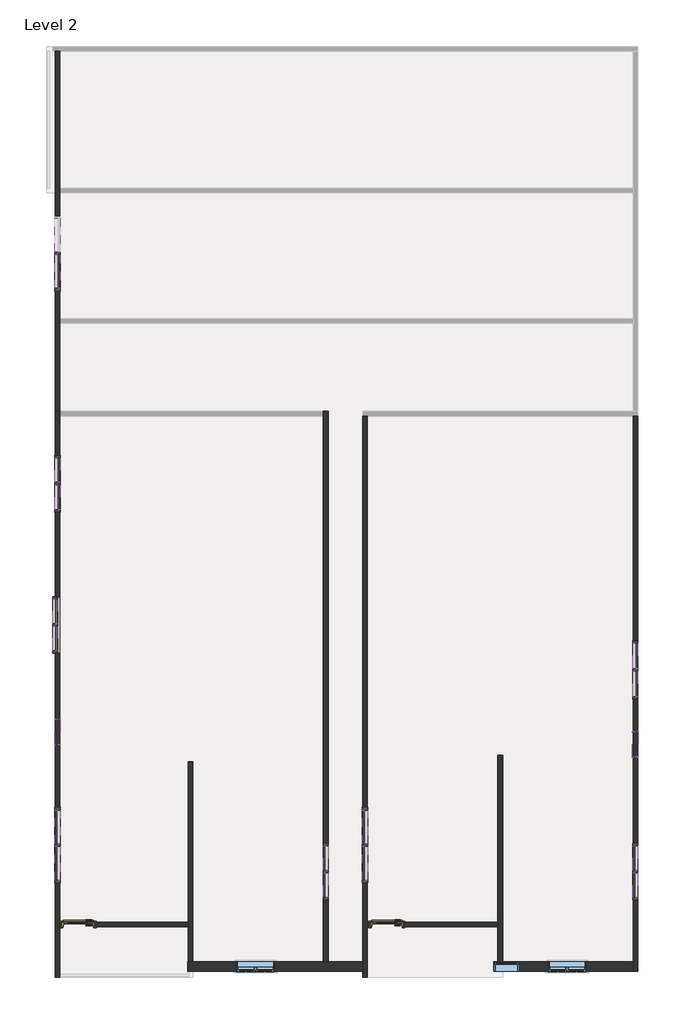
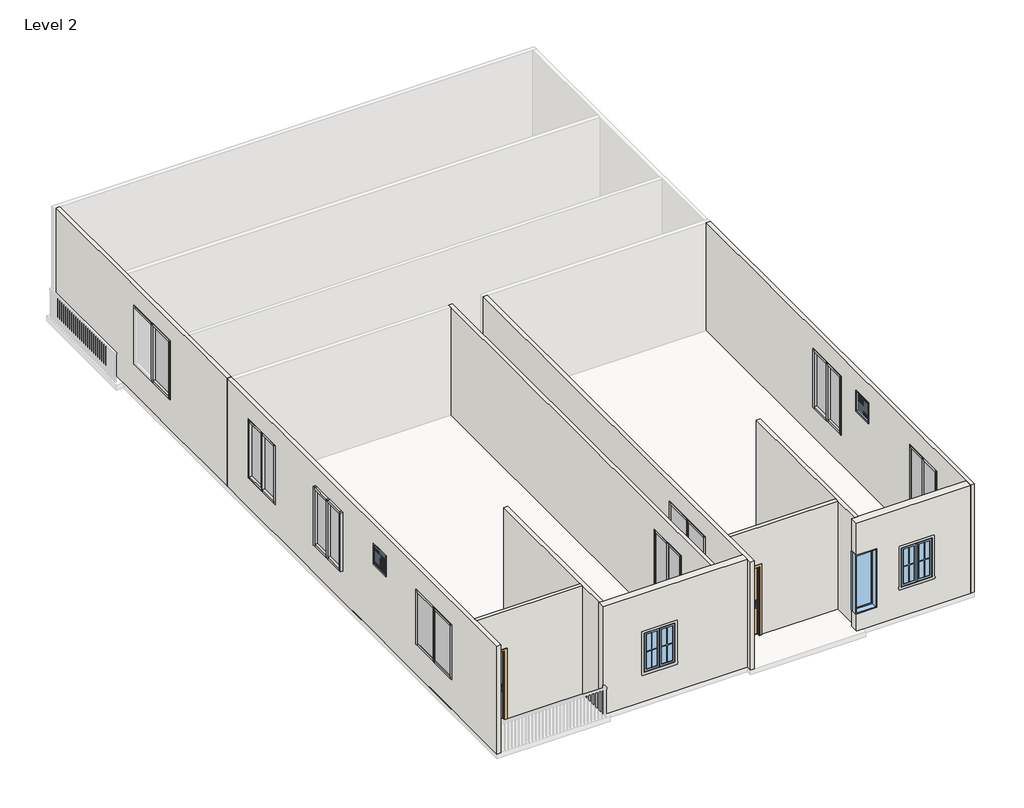
# One storey, part 1 of 2: 54 members, 15 plates, 11 walls, 5 windows, 2 doors.
"""IFC4 building model written with IfcOpenShell, lengths in millimetres."""

from ifc_helpers import new_model, si_unit, frame, origin, place, context, project, spatial, polyline, outline, extrude, faceted_brep, transform, mapped, element, save
from components import door_b81be692, member_8acf8d94, member_501b078b, member_3f0e0172, member_2e6d4a6b, member_96ae0c19, member_d60e8053, member_2fae0574, member_b8ac15de, member_17644e48, member_3e1d4a65, system_panel_glazed_c4393626, system_panel_glazed_0e71bc1b, system_panel_glazed_e97abd02, system_panel_glazed_d2c73f4b, system_panel_glazed_30879ba3, system_panel_glazed_a7ecbca6, window_fc882ab3, window_d341e8ac, window_d39e7ecb

model = new_model("IFC4")

# Units and contexts
model_context = context("Model", 3, world=origin())
ifc_project = project(units=[si_unit("LENGTHUNIT", "METRE", prefix="MILLI")], contexts=[model_context])

# Site, building, storey
site = spatial("IfcSite", under=ifc_project)
building = spatial("IfcBuilding", under=site)
storey = spatial("IfcBuildingStorey", under=building, Name="Level 2", Elevation=3352.8)

# Doors
placement = place(None, origin())
door_shape = door_b81be692(model_context)
element("IfcDoor", 1, ObjectType="29\" x 84\"", at=placement, inside=storey, context=model_context, shape_type="MappedRepresentation", body=[
    mapped(door_shape, transform((-7651.507583, -9448.7163489, 3352.8), x_axis=(1.0, 0.0, 0.0), y_axis=(0.0, 1.0, 0.0), z_axis=(0.0, 0.0, 1.0))),
])
element("IfcDoor", 2, ObjectType="29\" x 84\"", at=placement, inside=storey, context=model_context, shape_type="MappedRepresentation", body=[
    mapped(door_shape, transform((-172.2931282, -9448.9038009, 3352.8), x_axis=(1.0, 0.0, 0.0), y_axis=(0.0, 1.0, 0.0), z_axis=(0.0, 0.0, 1.0))),
])

# Members
member_shape = member_8acf8d94(model_context)
element("IfcMember", 3, ObjectType="Rectangular Mullion : 2.5\" x 5\" rectangular", at=placement, inside=storey, context=model_context, shape_type="MappedRepresentation", body=[
    mapped(member_shape, transform((-8153.157583, -8377.1401329, 5974.686558), x_axis=(0.0, 0.0, 1.0), y_axis=(-1.0, 0.0, 0.0), z_axis=(0.0, -1.0, 0.0))),
])
element("IfcMember", 4, ObjectType="Rectangular Mullion : 2.5\" x 5\" rectangular", at=placement, inside=storey, context=model_context, shape_type="MappedRepresentation", body=[
    mapped(member_shape, transform((-8153.157583, -7497.6651329, 5974.686558), x_axis=(0.0, 0.0, 1.0), y_axis=(-1.0, 0.0, 0.0), z_axis=(0.0, -1.0, 0.0))),
])
element("IfcMember", 5, ObjectType="Rectangular Mullion : 2.5\" x 5\" rectangular", at=placement, inside=storey, context=model_context, shape_type="MappedRepresentation", body=[
    mapped(member_shape, transform((-8153.157583, -6681.6901329, 4267.2), x_axis=(0.0, 0.0, -1.0), y_axis=(-1.0, 0.0, 0.0), z_axis=(0.0, 1.0, 0.0))),
])
element("IfcMember", 6, ObjectType="Rectangular Mullion : 2.5\" x 5\" rectangular", at=placement, inside=storey, context=model_context, shape_type="MappedRepresentation", body=[
    mapped(member_shape, transform((-8153.157583, -7561.1651329, 4267.2), x_axis=(0.0, 0.0, -1.0), y_axis=(-1.0, 0.0, 0.0), z_axis=(0.0, 1.0, 0.0))),
])
member_2_shape = member_501b078b(model_context)
element("IfcMember", 7, ObjectType="Rectangular Mullion : 2.5\" x 5\" rectangular", at=placement, inside=storey, context=model_context, shape_type="MappedRepresentation", body=[
    mapped(member_2_shape, transform((5848.1708786, -8795.0998253, 6096.0), x_axis=(0.0, 0.0, 1.0), y_axis=(-1.0, 0.0, 0.0), z_axis=(0.0, -1.0, 0.0))),
])
element("IfcMember", 8, ObjectType="Rectangular Mullion : 2.5\" x 5\" rectangular", at=placement, inside=storey, context=model_context, shape_type="MappedRepresentation", body=[
    mapped(member_2_shape, transform((5848.1708786, -8142.1745373, 6096.0), x_axis=(0.0, 0.0, 1.0), y_axis=(-1.0, 0.0, 0.0), z_axis=(0.0, -1.0, 0.0))),
])
element("IfcMember", 9, ObjectType="Rectangular Mullion : 2.5\" x 5\" rectangular", at=placement, inside=storey, context=model_context, shape_type="MappedRepresentation", body=[
    mapped(member_2_shape, transform((-1656.4435762, -8795.0998253, 6096.0), x_axis=(0.0, 0.0, 1.0), y_axis=(-1.0, 0.0, 0.0), z_axis=(0.0, -1.0, 0.0))),
])
element("IfcMember", 10, ObjectType="Rectangular Mullion : 2.5\" x 5\" rectangular", at=placement, inside=storey, context=model_context, shape_type="MappedRepresentation", body=[
    mapped(member_2_shape, transform((-1656.4435762, -8142.1745373, 6096.0), x_axis=(0.0, 0.0, 1.0), y_axis=(-1.0, 0.0, 0.0), z_axis=(0.0, -1.0, 0.0))),
])
element("IfcMember", 11, ObjectType="Rectangular Mullion : 2.5\" x 5\" rectangular", at=placement, inside=storey, context=model_context, shape_type="MappedRepresentation", body=[
    mapped(member_2_shape, transform((5848.1708786, -7552.7492493, 4267.2), x_axis=(0.0, 0.0, -1.0), y_axis=(-1.0, 0.0, 0.0), z_axis=(0.0, 1.0, 0.0))),
])
element("IfcMember", 12, ObjectType="Rectangular Mullion : 2.5\" x 5\" rectangular", at=placement, inside=storey, context=model_context, shape_type="MappedRepresentation", body=[
    mapped(member_2_shape, transform((5848.1708786, -8205.6745373, 4267.2), x_axis=(0.0, 0.0, -1.0), y_axis=(-1.0, 0.0, 0.0), z_axis=(0.0, 1.0, 0.0))),
])
element("IfcMember", 13, ObjectType="Rectangular Mullion : 2.5\" x 5\" rectangular", at=placement, inside=storey, context=model_context, shape_type="MappedRepresentation", body=[
    mapped(member_2_shape, transform((-1656.4435762, -7552.7492493, 4267.2), x_axis=(0.0, 0.0, -1.0), y_axis=(-1.0, 0.0, 0.0), z_axis=(0.0, 1.0, 0.0))),
])
element("IfcMember", 14, ObjectType="Rectangular Mullion : 2.5\" x 5\" rectangular", at=placement, inside=storey, context=model_context, shape_type="MappedRepresentation", body=[
    mapped(member_2_shape, transform((-1656.4435762, -8205.6745373, 4267.2), x_axis=(0.0, 0.0, -1.0), y_axis=(-1.0, 0.0, 0.0), z_axis=(0.0, 1.0, 0.0))),
])
member_3_shape = member_3f0e0172(model_context)
element("IfcMember", 15, ObjectType="Rectangular Mullion : 2.5\" x 5\" rectangular", at=placement, inside=storey, context=model_context, shape_type="MappedRepresentation", body=[
    mapped(member_3_shape, transform((5848.1708786, -3933.7021821, 6096.0), x_axis=(0.0, 0.0, 1.0), y_axis=(-1.0, 0.0, 0.0), z_axis=(0.0, -1.0, 0.0))),
])
element("IfcMember", 16, ObjectType="Rectangular Mullion : 2.5\" x 5\" rectangular", at=placement, inside=storey, context=model_context, shape_type="MappedRepresentation", body=[
    mapped(member_3_shape, transform((5848.1708786, -3254.2521821, 6096.0), x_axis=(0.0, 0.0, 1.0), y_axis=(-1.0, 0.0, 0.0), z_axis=(0.0, -1.0, 0.0))),
])
element("IfcMember", 17, ObjectType="Rectangular Mullion : 2.5\" x 5\" rectangular", at=placement, inside=storey, context=model_context, shape_type="MappedRepresentation", body=[
    mapped(member_3_shape, transform((5848.1708786, -2638.3021821, 4267.2), x_axis=(0.0, 0.0, -1.0), y_axis=(-1.0, 0.0, 0.0), z_axis=(0.0, 1.0, 0.0))),
])
element("IfcMember", 18, ObjectType="Rectangular Mullion : 2.5\" x 5\" rectangular", at=placement, inside=storey, context=model_context, shape_type="MappedRepresentation", body=[
    mapped(member_3_shape, transform((5848.1708786, -3317.7521821, 4267.2), x_axis=(0.0, 0.0, -1.0), y_axis=(-1.0, 0.0, 0.0), z_axis=(0.0, 1.0, 0.0))),
])
member_4_shape = member_2e6d4a6b(model_context)
element("IfcMember", 19, ObjectType="Rectangular Mullion : 2.5\" x 5\" rectangular", at=placement, inside=storey, context=model_context, shape_type="MappedRepresentation", body=[
    mapped(member_4_shape, transform((-705.6931282, -8380.4909009, 6096.0), x_axis=(0.0, 0.0, 1.0), y_axis=(-1.0, 0.0, 0.0), z_axis=(0.0, -1.0, 0.0))),
])
element("IfcMember", 20, ObjectType="Rectangular Mullion : 2.5\" x 5\" rectangular", at=placement, inside=storey, context=model_context, shape_type="MappedRepresentation", body=[
    mapped(member_4_shape, transform((-705.6931282, -7499.3405169, 6096.0), x_axis=(0.0, 0.0, 1.0), y_axis=(-1.0, 0.0, 0.0), z_axis=(0.0, -1.0, 0.0))),
])
element("IfcMember", 21, ObjectType="Rectangular Mullion : 2.5\" x 5\" rectangular", at=placement, inside=storey, context=model_context, shape_type="MappedRepresentation", body=[
    mapped(member_4_shape, transform((-705.6931282, -6681.6901329, 4267.2), x_axis=(0.0, 0.0, -1.0), y_axis=(-1.0, 0.0, 0.0), z_axis=(0.0, 1.0, 0.0))),
])
element("IfcMember", 22, ObjectType="Rectangular Mullion : 2.5\" x 5\" rectangular", at=placement, inside=storey, context=model_context, shape_type="MappedRepresentation", body=[
    mapped(member_4_shape, transform((-705.6931282, -7562.8405169, 4267.2), x_axis=(0.0, 0.0, -1.0), y_axis=(-1.0, 0.0, 0.0), z_axis=(0.0, 1.0, 0.0))),
])
member_5_shape = member_96ae0c19(model_context)
element("IfcMember", 23, ObjectType="Rectangular Mullion : 2.5\" x 5\" rectangular", at=placement, inside=storey, context=model_context, shape_type="MappedRepresentation", body=[
    mapped(member_5_shape, transform((-8153.157583, 600.1666267, 6096.0), x_axis=(0.0, 0.0, 1.0), y_axis=(-1.0, 0.0, 0.0), z_axis=(0.0, -1.0, 0.0))),
])
element("IfcMember", 24, ObjectType="Rectangular Mullion : 2.5\" x 5\" rectangular", at=placement, inside=storey, context=model_context, shape_type="MappedRepresentation", body=[
    mapped(member_5_shape, transform((-8153.157583, 1254.9937905, 6096.0), x_axis=(0.0, 0.0, 1.0), y_axis=(-1.0, 0.0, 0.0), z_axis=(0.0, -1.0, 0.0))),
])
element("IfcMember", 25, ObjectType="Rectangular Mullion : 2.5\" x 5\" rectangular", at=placement, inside=storey, context=model_context, shape_type="MappedRepresentation", body=[
    mapped(member_5_shape, transform((-8210.307583, -2819.4060617, 6096.0), x_axis=(0.0, 0.0, 1.0), y_axis=(-1.0, 0.0, 0.0), z_axis=(0.0, -1.0, 0.0))),
])
element("IfcMember", 26, ObjectType="Rectangular Mullion : 2.5\" x 5\" rectangular", at=placement, inside=storey, context=model_context, shape_type="MappedRepresentation", body=[
    mapped(member_5_shape, transform((-8210.307583, -2164.5788979, 6096.0), x_axis=(0.0, 0.0, 1.0), y_axis=(-1.0, 0.0, 0.0), z_axis=(0.0, -1.0, 0.0))),
])
element("IfcMember", 27, ObjectType="Rectangular Mullion : 2.5\" x 5\" rectangular", at=placement, inside=storey, context=model_context, shape_type="MappedRepresentation", body=[
    mapped(member_5_shape, transform((-8153.157583, 1846.3209543, 4267.2), x_axis=(0.0, 0.0, -1.0), y_axis=(-1.0, 0.0, 0.0), z_axis=(0.0, 1.0, 0.0))),
])
element("IfcMember", 28, ObjectType="Rectangular Mullion : 2.5\" x 5\" rectangular", at=placement, inside=storey, context=model_context, shape_type="MappedRepresentation", body=[
    mapped(member_5_shape, transform((-8153.157583, 1191.4937905, 4267.2), x_axis=(0.0, 0.0, -1.0), y_axis=(-1.0, 0.0, 0.0), z_axis=(0.0, 1.0, 0.0))),
])
element("IfcMember", 29, ObjectType="Rectangular Mullion : 2.5\" x 5\" rectangular", at=placement, inside=storey, context=model_context, shape_type="MappedRepresentation", body=[
    mapped(member_5_shape, transform((-8210.307583, -1573.2517341, 4267.2), x_axis=(0.0, 0.0, -1.0), y_axis=(-1.0, 0.0, 0.0), z_axis=(0.0, 1.0, 0.0))),
])
element("IfcMember", 30, ObjectType="Rectangular Mullion : 2.5\" x 5\" rectangular", at=placement, inside=storey, context=model_context, shape_type="MappedRepresentation", body=[
    mapped(member_5_shape, transform((-8210.307583, -2228.0788979, 4267.2), x_axis=(0.0, 0.0, -1.0), y_axis=(-1.0, 0.0, 0.0), z_axis=(0.0, 1.0, 0.0))),
])
member_6_shape = member_d60e8053(model_context)
element("IfcMember", 31, ObjectType="Rectangular Mullion : 2.5\" x 5\" rectangular", at=placement, inside=storey, context=model_context, shape_type="MappedRepresentation", body=[
    mapped(member_6_shape, transform((5848.1708786, -3286.0021821, 4267.2), x_axis=(0.0, -1.0, 0.0), y_axis=(-1.0, 0.0, 0.0), z_axis=(0.0, 0.0, -1.0))),
])
element("IfcMember", 32, ObjectType="Rectangular Mullion : 2.5\" x 5\" rectangular", at=placement, inside=storey, context=model_context, shape_type="MappedRepresentation", body=[
    mapped(member_6_shape, transform((-8153.157583, 1223.2437905, 4267.2), x_axis=(0.0, -1.0, 0.0), y_axis=(-1.0, 0.0, 0.0), z_axis=(0.0, 0.0, -1.0))),
])
element("IfcMember", 33, ObjectType="Rectangular Mullion : 2.5\" x 5\" rectangular", at=placement, inside=storey, context=model_context, shape_type="MappedRepresentation", body=[
    mapped(member_6_shape, transform((-8210.307583, -2196.3288979, 4267.2), x_axis=(0.0, -1.0, 0.0), y_axis=(-1.0, 0.0, 0.0), z_axis=(0.0, 0.0, -1.0))),
])
element("IfcMember", 34, ObjectType="Rectangular Mullion : 2.5\" x 5\" rectangular", at=placement, inside=storey, context=model_context, shape_type="MappedRepresentation", body=[
    mapped(member_6_shape, transform((-8153.157583, 6807.1511393, 4267.2), x_axis=(0.0, -1.0, 0.0), y_axis=(-1.0, 0.0, 0.0), z_axis=(0.0, 0.0, -1.0))),
])
member_7_shape = member_2fae0574(model_context)
element("IfcMember", 35, ObjectType="Rectangular Mullion : 2.5\" x 5\" rectangular", at=placement, inside=storey, context=model_context, shape_type="MappedRepresentation", body=[
    mapped(member_7_shape, transform((5848.1708786, -2574.8021821, 6096.0), x_axis=(0.0, 1.0, 0.0), y_axis=(-1.0, 0.0, 0.0), z_axis=(0.0, 0.0, 1.0))),
])
element("IfcMember", 36, ObjectType="Rectangular Mullion : 2.5\" x 5\" rectangular", at=placement, inside=storey, context=model_context, shape_type="MappedRepresentation", body=[
    mapped(member_7_shape, transform((-8153.157583, 1909.8209543, 6096.0), x_axis=(0.0, 1.0, 0.0), y_axis=(-1.0, 0.0, 0.0), z_axis=(0.0, 0.0, 1.0))),
])
element("IfcMember", 37, ObjectType="Rectangular Mullion : 2.5\" x 5\" rectangular", at=placement, inside=storey, context=model_context, shape_type="MappedRepresentation", body=[
    mapped(member_7_shape, transform((-8210.307583, -1509.7517341, 6096.0), x_axis=(0.0, 1.0, 0.0), y_axis=(-1.0, 0.0, 0.0), z_axis=(0.0, 0.0, 1.0))),
])
element("IfcMember", 38, ObjectType="Rectangular Mullion : 2.5\" x 5\" rectangular", at=placement, inside=storey, context=model_context, shape_type="MappedRepresentation", body=[
    mapped(member_7_shape, transform((5848.1708786, -3997.2021821, 4267.2), x_axis=(0.0, -1.0, 0.0), y_axis=(-1.0, 0.0, 0.0), z_axis=(0.0, 0.0, -1.0))),
])
element("IfcMember", 39, ObjectType="Rectangular Mullion : 2.5\" x 5\" rectangular", at=placement, inside=storey, context=model_context, shape_type="MappedRepresentation", body=[
    mapped(member_7_shape, transform((-8153.157583, 536.6666267, 4267.2), x_axis=(0.0, -1.0, 0.0), y_axis=(-1.0, 0.0, 0.0), z_axis=(0.0, 0.0, -1.0))),
])
element("IfcMember", 40, ObjectType="Rectangular Mullion : 2.5\" x 5\" rectangular", at=placement, inside=storey, context=model_context, shape_type="MappedRepresentation", body=[
    mapped(member_7_shape, transform((-8210.307583, -2882.9060617, 4267.2), x_axis=(0.0, -1.0, 0.0), y_axis=(-1.0, 0.0, 0.0), z_axis=(0.0, 0.0, -1.0))),
])
element("IfcMember", 41, ObjectType="Rectangular Mullion : 2.5\" x 5\" rectangular", at=placement, inside=storey, context=model_context, shape_type="MappedRepresentation", body=[
    mapped(member_7_shape, transform((-8153.157583, 5892.3488795, 4267.2), x_axis=(0.0, -1.0, 0.0), y_axis=(-1.0, 0.0, 0.0), z_axis=(0.0, 0.0, -1.0))),
])
member_8_shape = member_b8ac15de(model_context)
element("IfcMember", 42, ObjectType="Rectangular Mullion : 2.5\" x 5\" rectangular", at=placement, inside=storey, context=model_context, shape_type="MappedRepresentation", body=[
    mapped(member_8_shape, transform((-8153.157583, -7529.4151329, 4267.2), x_axis=(0.0, -1.0, 0.0), y_axis=(-1.0, 0.0, 0.0), z_axis=(0.0, 0.0, -1.0))),
])
member_9_shape = member_17644e48(model_context)
element("IfcMember", 43, ObjectType="Rectangular Mullion : 2.5\" x 5\" rectangular", at=placement, inside=storey, context=model_context, shape_type="MappedRepresentation", body=[
    mapped(member_9_shape, transform((-8153.157583, -6618.1901329, 5974.686558), x_axis=(0.0, 1.0, 0.0), y_axis=(-1.0, 0.0, 0.0), z_axis=(0.0, 0.0, 1.0))),
])
element("IfcMember", 44, ObjectType="Rectangular Mullion : 2.5\" x 5\" rectangular", at=placement, inside=storey, context=model_context, shape_type="MappedRepresentation", body=[
    mapped(member_9_shape, transform((-8153.157583, -8440.6401329, 4267.2), x_axis=(0.0, -1.0, 0.0), y_axis=(-1.0, 0.0, 0.0), z_axis=(0.0, 0.0, -1.0))),
])
element("IfcMember", 45, ObjectType="Rectangular Mullion : 2.5\" x 5\" rectangular", at=placement, inside=storey, context=model_context, shape_type="MappedRepresentation", body=[
    mapped(member_6_shape, transform((5848.1708786, -8173.9245373, 4267.2), x_axis=(0.0, -1.0, 0.0), y_axis=(-1.0, 0.0, 0.0), z_axis=(0.0, 0.0, -1.0))),
])
element("IfcMember", 46, ObjectType="Rectangular Mullion : 2.5\" x 5\" rectangular", at=placement, inside=storey, context=model_context, shape_type="MappedRepresentation", body=[
    mapped(member_6_shape, transform((-1656.4435762, -8173.9245373, 4267.2), x_axis=(0.0, -1.0, 0.0), y_axis=(-1.0, 0.0, 0.0), z_axis=(0.0, 0.0, -1.0))),
])
element("IfcMember", 47, ObjectType="Rectangular Mullion : 2.5\" x 5\" rectangular", at=placement, inside=storey, context=model_context, shape_type="MappedRepresentation", body=[
    mapped(member_6_shape, transform((-705.6931282, -7531.0905169, 4267.2), x_axis=(0.0, -1.0, 0.0), y_axis=(-1.0, 0.0, 0.0), z_axis=(0.0, 0.0, -1.0))),
])
element("IfcMember", 48, ObjectType="Rectangular Mullion : 2.5\" x 5\" rectangular", at=placement, inside=storey, context=model_context, shape_type="MappedRepresentation", body=[
    mapped(member_7_shape, transform((5848.1708786, -7489.2492493, 6096.0), x_axis=(0.0, 1.0, 0.0), y_axis=(-1.0, 0.0, 0.0), z_axis=(0.0, 0.0, 1.0))),
])
element("IfcMember", 49, ObjectType="Rectangular Mullion : 2.5\" x 5\" rectangular", at=placement, inside=storey, context=model_context, shape_type="MappedRepresentation", body=[
    mapped(member_7_shape, transform((-1656.4435762, -7489.2492493, 6096.0), x_axis=(0.0, 1.0, 0.0), y_axis=(-1.0, 0.0, 0.0), z_axis=(0.0, 0.0, 1.0))),
])
element("IfcMember", 50, ObjectType="Rectangular Mullion : 2.5\" x 5\" rectangular", at=placement, inside=storey, context=model_context, shape_type="MappedRepresentation", body=[
    mapped(member_7_shape, transform((-705.6931282, -6618.1901329, 6096.0), x_axis=(0.0, 1.0, 0.0), y_axis=(-1.0, 0.0, 0.0), z_axis=(0.0, 0.0, 1.0))),
])
element("IfcMember", 51, ObjectType="Rectangular Mullion : 2.5\" x 5\" rectangular", at=placement, inside=storey, context=model_context, shape_type="MappedRepresentation", body=[
    mapped(member_7_shape, transform((5848.1708786, -8858.5998253, 4267.2), x_axis=(0.0, -1.0, 0.0), y_axis=(-1.0, 0.0, 0.0), z_axis=(0.0, 0.0, -1.0))),
])
element("IfcMember", 52, ObjectType="Rectangular Mullion : 2.5\" x 5\" rectangular", at=placement, inside=storey, context=model_context, shape_type="MappedRepresentation", body=[
    mapped(member_7_shape, transform((-1656.4435762, -8858.5998253, 4267.2), x_axis=(0.0, -1.0, 0.0), y_axis=(-1.0, 0.0, 0.0), z_axis=(0.0, 0.0, -1.0))),
])
element("IfcMember", 53, ObjectType="Rectangular Mullion : 2.5\" x 5\" rectangular", at=placement, inside=storey, context=model_context, shape_type="MappedRepresentation", body=[
    mapped(member_7_shape, transform((-705.6931282, -8443.9909009, 4267.2), x_axis=(0.0, -1.0, 0.0), y_axis=(-1.0, 0.0, 0.0), z_axis=(0.0, 0.0, -1.0))),
])
member_10_shape = member_3e1d4a65(model_context)
element("IfcMember", 54, ObjectType="Rectangular Mullion : 2.5\" x 5\" rectangular", at=placement, inside=storey, context=model_context, shape_type="MappedRepresentation", body=[
    mapped(member_10_shape, transform((-8153.157583, 5955.8488795, 6096.0), x_axis=(0.0, 0.0, 1.0), y_axis=(-1.0, 0.0, 0.0), z_axis=(0.0, -1.0, 0.0))),
])
element("IfcMember", 55, ObjectType="Rectangular Mullion : 2.5\" x 5\" rectangular", at=placement, inside=storey, context=model_context, shape_type="MappedRepresentation", body=[
    mapped(member_10_shape, transform((-8153.157583, 6838.9011393, 6096.0), x_axis=(0.0, 0.0, 1.0), y_axis=(-1.0, 0.0, 0.0), z_axis=(0.0, -1.0, 0.0))),
])
element("IfcMember", 56, ObjectType="Rectangular Mullion : 2.5\" x 5\" rectangular", at=placement, inside=storey, context=model_context, shape_type="MappedRepresentation", body=[
    mapped(member_10_shape, transform((-8153.157583, 6775.4011393, 4267.2), x_axis=(0.0, 0.0, -1.0), y_axis=(-1.0, 0.0, 0.0), z_axis=(0.0, 1.0, 0.0))),
])

# Plates
system_panel_glazed_shape = system_panel_glazed_c4393626(model_context)
element("IfcPlate", 57, ObjectType="System Panel : Glazed", at=placement, inside=storey, context=model_context, shape_type="MappedRepresentation", body=[
    mapped(system_panel_glazed_shape, transform((-8210.307583, -1868.915316, 4330.7), x_axis=(0.0, -1.0, 0.0), y_axis=(1.0, 0.0, 0.0), z_axis=(0.0, 0.0, 1.0))),
])
element("IfcPlate", 58, ObjectType="System Panel : Glazed", at=placement, inside=storey, context=model_context, shape_type="MappedRepresentation", body=[
    mapped(system_panel_glazed_shape, transform((-8153.157583, 1550.6573724, 4330.7), x_axis=(0.0, -1.0, 0.0), y_axis=(1.0, 0.0, 0.0), z_axis=(0.0, 0.0, 1.0))),
])
element("IfcPlate", 59, ObjectType="System Panel : Glazed", at=placement, inside=storey, context=model_context, shape_type="MappedRepresentation", body=[
    mapped(system_panel_glazed_shape, transform((-8153.157583, 895.8302086, 4330.7), x_axis=(0.0, -1.0, 0.0), y_axis=(1.0, 0.0, 0.0), z_axis=(0.0, 0.0, 1.0))),
])
element("IfcPlate", 60, ObjectType="System Panel : Glazed", at=placement, inside=storey, context=model_context, shape_type="MappedRepresentation", body=[
    mapped(system_panel_glazed_shape, transform((-8210.307583, -2523.7424798, 4330.7), x_axis=(0.0, -1.0, 0.0), y_axis=(1.0, 0.0, 0.0), z_axis=(0.0, 0.0, 1.0))),
])
system_panel_glazed_2_shape = system_panel_glazed_0e71bc1b(model_context)
element("IfcPlate", 61, ObjectType="System Panel : Glazed", at=placement, inside=storey, context=model_context, shape_type="MappedRepresentation", body=[
    mapped(system_panel_glazed_2_shape, transform((-8153.157583, -7089.6776329, 4330.7), x_axis=(0.0, -1.0, 0.0), y_axis=(1.0, 0.0, 0.0), z_axis=(0.0, 0.0, 1.0))),
])
element("IfcPlate", 62, ObjectType="System Panel : Glazed", at=placement, inside=storey, context=model_context, shape_type="MappedRepresentation", body=[
    mapped(system_panel_glazed_2_shape, transform((-8153.157583, -7969.1526329, 4330.7), x_axis=(0.0, -1.0, 0.0), y_axis=(1.0, 0.0, 0.0), z_axis=(0.0, 0.0, 1.0))),
])
system_panel_glazed_3_shape = system_panel_glazed_e97abd02(model_context)
element("IfcPlate", 63, ObjectType="System Panel : Glazed", at=placement, inside=storey, context=model_context, shape_type="MappedRepresentation", body=[
    mapped(system_panel_glazed_3_shape, transform((5848.1708786, -7847.4618933, 4330.7), x_axis=(0.0, -1.0, 0.0), y_axis=(1.0, 0.0, 0.0), z_axis=(0.0, 0.0, 1.0))),
])
element("IfcPlate", 64, ObjectType="System Panel : Glazed", at=placement, inside=storey, context=model_context, shape_type="MappedRepresentation", body=[
    mapped(system_panel_glazed_3_shape, transform((-1656.4435762, -7847.4618933, 4330.7), x_axis=(0.0, -1.0, 0.0), y_axis=(1.0, 0.0, 0.0), z_axis=(0.0, 0.0, 1.0))),
])
element("IfcPlate", 65, ObjectType="System Panel : Glazed", at=placement, inside=storey, context=model_context, shape_type="MappedRepresentation", body=[
    mapped(system_panel_glazed_3_shape, transform((5848.1708786, -8500.3871813, 4330.7), x_axis=(0.0, -1.0, 0.0), y_axis=(1.0, 0.0, 0.0), z_axis=(0.0, 0.0, 1.0))),
])
element("IfcPlate", 66, ObjectType="System Panel : Glazed", at=placement, inside=storey, context=model_context, shape_type="MappedRepresentation", body=[
    mapped(system_panel_glazed_3_shape, transform((-1656.4435762, -8500.3871813, 4330.7), x_axis=(0.0, -1.0, 0.0), y_axis=(1.0, 0.0, 0.0), z_axis=(0.0, 0.0, 1.0))),
])
system_panel_glazed_4_shape = system_panel_glazed_d2c73f4b(model_context)
element("IfcPlate", 67, ObjectType="System Panel : Glazed", at=placement, inside=storey, context=model_context, shape_type="MappedRepresentation", body=[
    mapped(system_panel_glazed_4_shape, transform((5848.1708786, -2946.2771821, 4330.7), x_axis=(0.0, -1.0, 0.0), y_axis=(1.0, 0.0, 0.0), z_axis=(0.0, 0.0, 1.0))),
])
element("IfcPlate", 68, ObjectType="System Panel : Glazed", at=placement, inside=storey, context=model_context, shape_type="MappedRepresentation", body=[
    mapped(system_panel_glazed_4_shape, transform((5848.1708786, -3625.7271821, 4330.7), x_axis=(0.0, -1.0, 0.0), y_axis=(1.0, 0.0, 0.0), z_axis=(0.0, 0.0, 1.0))),
])
system_panel_glazed_5_shape = system_panel_glazed_30879ba3(model_context)
element("IfcPlate", 69, ObjectType="System Panel : Glazed", at=placement, inside=storey, context=model_context, shape_type="MappedRepresentation", body=[
    mapped(system_panel_glazed_5_shape, transform((-8153.157583, 6365.6250094, 4330.7), x_axis=(0.0, -1.0, 0.0), y_axis=(1.0, 0.0, 0.0), z_axis=(0.0, 0.0, 1.0))),
])
system_panel_glazed_6_shape = system_panel_glazed_a7ecbca6(model_context)
element("IfcPlate", 70, ObjectType="System Panel : Glazed", at=placement, inside=storey, context=model_context, shape_type="MappedRepresentation", body=[
    mapped(system_panel_glazed_6_shape, transform((-705.6931282, -7090.5153249, 4330.7), x_axis=(0.0, -1.0, 0.0), y_axis=(1.0, 0.0, 0.0), z_axis=(0.0, 0.0, 1.0))),
])
element("IfcPlate", 71, ObjectType="System Panel : Glazed", at=placement, inside=storey, context=model_context, shape_type="MappedRepresentation", body=[
    mapped(system_panel_glazed_6_shape, transform((-705.6931282, -7971.6657089, 4330.7), x_axis=(0.0, -1.0, 0.0), y_axis=(1.0, 0.0, 0.0), z_axis=(0.0, 0.0, 1.0))),
])

# Walls
element("IfcWall", 72, ObjectType="4.5\" wall", at=placement, inside=storey, context=model_context, shape_type="Brep", body=[
    faceted_brep([(-8096.007583, -10738.0280197, 3352.8), (-8096.007583, -9509.0413489, 3352.8), (-8096.007583, -9394.7413489, 3352.8), (-8096.007583, 2864.0002499, 3352.8), (-8096.007583, 2978.3002499, 3352.8), (-8096.007583, 2978.3002499, 6705.6), (-8096.007583, 2864.0002499, 6705.6), (-8096.007583, -9394.7413489, 6705.6), (-8096.007583, -9509.0413489, 6705.6), (-8096.007583, -10738.0280197, 6705.6), (-8096.007583, -6618.1901329, 5974.686558), (-8096.007583, -6618.1901329, 4267.2), (-8096.007583, -8440.6401329, 4267.2), (-8096.007583, -8440.6401329, 5974.686558), (-8096.007583, -5094.1901329, 5467.35), (-8096.007583, -5094.1901329, 6076.95), (-8096.007583, -4484.5901329, 6076.95), (-8096.007583, -4484.5901329, 5467.35), (-8096.007583, 1909.8209543, 6096.0), (-8096.007583, 1909.8209543, 4267.2), (-8096.007583, 536.6666267, 4267.2), (-8096.007583, 536.6666267, 6096.0), (-8096.007583, -1509.7517341, 6096.0), (-8096.007583, -1509.7517341, 4267.2), (-8096.007583, -2882.9060617, 4267.2), (-8096.007583, -2882.9060617, 6096.0), (-8210.307583, 2978.3002499, 3352.8), (-8210.307583, -10738.0280197, 3352.8), (-8210.307583, -10738.0280197, 6705.6), (-8210.307583, 2978.3002499, 6705.6), (-8210.307583, -6618.1901329, 4267.2), (-8210.307583, -6618.1901329, 5974.686558), (-8210.307583, -8440.6401329, 5974.686558), (-8210.307583, -8440.6401329, 4267.2), (-8210.307583, -5094.1901329, 6076.95), (-8210.307583, -5094.1901329, 5467.35), (-8210.307583, -4484.5901329, 5467.35), (-8210.307583, -4484.5901329, 6076.95), (-8210.307583, 1909.8209543, 4267.2), (-8210.307583, 1909.8209543, 6096.0), (-8210.307583, 536.6666267, 6096.0), (-8210.307583, 536.6666267, 4267.2), (-8210.307583, -1509.7517341, 4267.2), (-8210.307583, -1509.7517341, 6096.0), (-8210.307583, -2882.9060617, 6096.0), (-8210.307583, -2882.9060617, 4267.2)], [[[0, 1, 2, 3, 4, 5, 6, 7, 8, 9], [10, 11, 12, 13], [14, 15, 16, 17], [18, 19, 20, 21], [22, 23, 24, 25]], [[26, 27, 28, 29], [30, 31, 32, 33], [34, 35, 36, 37], [38, 39, 40, 41], [42, 43, 44, 45]], [[4, 3, 2, 1, 0, 27, 26]], [[9, 8, 7, 6, 5, 29, 28]], [[0, 9, 28, 27]], [[5, 4, 26, 29]], [[10, 31, 30, 11]], [[31, 10, 13, 32]], [[32, 13, 12, 33]], [[11, 30, 33, 12]], [[35, 34, 15, 14]], [[36, 35, 14, 17]], [[37, 36, 17, 16]], [[34, 37, 16, 15]], [[38, 19, 18, 39]], [[39, 18, 21, 40]], [[40, 21, 20, 41]], [[19, 38, 41, 20]], [[22, 43, 42, 23]], [[43, 22, 25, 44]], [[44, 25, 24, 45]], [[23, 42, 45, 24]]]),
])
element("IfcWall", 73, ObjectType="4.5\" wall", at=placement, inside=storey, context=model_context, shape_type="Brep", body=[
    faceted_brep([(-1599.2935762, -10357.2779557, 3352.8), (-1599.2935762, 2978.3002499, 3352.8), (-1599.2935762, 2978.3002499, 6705.6), (-1599.2935762, -10357.2779557, 6705.6), (-1599.2935762, -7489.2492493, 6096.0), (-1599.2935762, -7489.2492493, 4267.2), (-1599.2935762, -8858.5998253, 4267.2), (-1599.2935762, -8858.5998253, 6096.0), (-1713.5935762, 2978.3002499, 3352.8), (-1713.5935762, 2864.0002499, 3352.8), (-1713.5935762, -10357.2779557, 3352.8), (-1713.5935762, -10357.2779557, 6705.6), (-1713.5935762, 2864.0002499, 6705.6), (-1713.5935762, 2978.3002499, 6705.6), (-1713.5935762, -7489.2492493, 4267.2), (-1713.5935762, -7489.2492493, 6096.0), (-1713.5935762, -8858.5998253, 6096.0), (-1713.5935762, -8858.5998253, 4267.2)], [[[0, 1, 2, 3], [4, 5, 6, 7]], [[8, 9, 10, 11, 12, 13], [14, 15, 16, 17]], [[1, 0, 10, 9, 8]], [[3, 2, 13, 12, 11]], [[2, 1, 8, 13]], [[0, 3, 11, 10]], [[14, 5, 4, 15]], [[15, 4, 7, 16]], [[16, 7, 6, 17]], [[5, 14, 17, 6]]]),
])
element("IfcWall", 74, ObjectType="4.5\" wall", at=placement, inside=storey, context=model_context, shape_type="Brep", body=[
    faceted_brep([(-8096.007583, 2978.3002499, 3352.8), (-8096.007583, 5112.2048975, 3352.8), (-8096.007583, 5226.5048975, 3352.8), (-8096.007583, 8273.1224771, 3352.8), (-8096.007583, 8387.4224771, 3352.8), (-8096.007583, 11703.9189683, 3352.8), (-8096.007583, 11703.9189683, 6705.6), (-8096.007583, 8387.4224771, 6705.6), (-8096.007583, 8273.1224771, 6705.6), (-8096.007583, 5226.5048975, 6705.6), (-8096.007583, 5112.2048975, 6705.6), (-8096.007583, 2978.3002499, 6705.6), (-8096.007583, 7721.9533991, 6096.0), (-8096.007583, 7721.9533991, 4267.2), (-8096.007583, 5892.3488795, 4267.2), (-8096.007583, 5892.3488795, 6096.0), (-8210.307583, 11703.9189683, 3352.8), (-8210.307583, 2978.3002499, 3352.8), (-8210.307583, 2978.3002499, 6705.6), (-8210.307583, 11703.9189683, 6705.6), (-8210.307583, 7721.9533991, 4267.2), (-8210.307583, 7721.9533991, 6096.0), (-8210.307583, 5892.3488795, 6096.0), (-8210.307583, 5892.3488795, 4267.2)], [[[0, 1, 2, 3, 4, 5, 6, 7, 8, 9, 10, 11], [12, 13, 14, 15]], [[16, 17, 18, 19], [20, 21, 22, 23]], [[5, 4, 3, 2, 1, 0, 17, 16]], [[11, 10, 9, 8, 7, 6, 19, 18]], [[6, 5, 16, 19]], [[0, 11, 18, 17]], [[20, 13, 12, 21]], [[21, 12, 15, 22]], [[22, 15, 14, 23]], [[13, 20, 23, 14]]]),
])
element("IfcWall", 75, ObjectType="4.5\" wall", at=placement, inside=storey, context=model_context, shape_type="Brep", body=[
    faceted_brep([(5791.0208786, 2864.0002499, 3352.8), (5791.0208786, -10357.2779557, 3352.8), (5791.0208786, -10585.8779557, 3352.8), (5791.0208786, -10585.8779557, 6705.6), (5791.0208786, -10357.2779557, 6705.6), (5791.0208786, 2864.0002499, 6705.6), (5791.0208786, -7489.2492493, 4267.2), (5791.0208786, -7489.2492493, 6096.0), (5791.0208786, -8858.5998253, 6096.0), (5791.0208786, -8858.5998253, 4267.2), (5791.0208786, -2574.8021821, 4267.2), (5791.0208786, -2574.8021821, 6096.0), (5791.0208786, -3997.2021821, 6096.0), (5791.0208786, -3997.2021821, 4267.2), (5791.0208786, -4784.6021821, 5505.45), (5791.0208786, -4784.6021821, 6115.05), (5791.0208786, -5394.2021821, 6115.05), (5791.0208786, -5394.2021821, 5505.45), (5905.3208786, -10585.8779557, 3352.8), (5905.3208786, 2864.0002499, 3352.8), (5905.3208786, 2864.0002499, 6705.6), (5905.3208786, -10585.8779557, 6705.6), (5905.3208786, -7489.2492493, 6096.0), (5905.3208786, -7489.2492493, 4267.2), (5905.3208786, -8858.5998253, 4267.2), (5905.3208786, -8858.5998253, 6096.0), (5905.3208786, -2574.8021821, 6096.0), (5905.3208786, -2574.8021821, 4267.2), (5905.3208786, -3997.2021821, 4267.2), (5905.3208786, -3997.2021821, 6096.0), (5905.3208786, -4784.6021821, 6115.05), (5905.3208786, -4784.6021821, 5505.45), (5905.3208786, -5394.2021821, 5505.45), (5905.3208786, -5394.2021821, 6115.05)], [[[0, 1, 2, 3, 4, 5], [6, 7, 8, 9], [10, 11, 12, 13], [14, 15, 16, 17]], [[18, 19, 20, 21], [22, 23, 24, 25], [26, 27, 28, 29], [30, 31, 32, 33]], [[2, 1, 0, 19, 18]], [[5, 4, 3, 21, 20]], [[0, 5, 20, 19]], [[3, 2, 18, 21]], [[22, 7, 6, 23]], [[7, 22, 25, 8]], [[8, 25, 24, 9]], [[23, 6, 9, 24]], [[10, 27, 26, 11]], [[11, 26, 29, 12]], [[12, 29, 28, 13]], [[27, 10, 13, 28]], [[31, 30, 15, 14]], [[32, 31, 14, 17]], [[33, 32, 17, 16]], [[30, 33, 16, 15]]]),
])
element("IfcWall", 76, ObjectType="4.5\" wall", at=placement, inside=storey, context=model_context, shape_type="Brep", body=[
    faceted_brep([(-762.8431282, 2864.0002499, 3352.8), (-762.8431282, -10357.2779557, 3352.8), (-762.8431282, -10585.8779557, 3352.8), (-762.8431282, -10737.6531157, 3352.8), (-762.8431282, -10737.6531157, 6705.6), (-762.8431282, -10585.8779557, 6705.6), (-762.8431282, -10357.2779557, 6705.6), (-762.8431282, 2864.0002499, 6705.6), (-762.8431282, -6618.1901329, 4267.2), (-762.8431282, -6618.1901329, 6096.0), (-762.8431282, -8443.9909009, 6096.0), (-762.8431282, -8443.9909009, 4267.2), (-648.5431282, -10737.6531157, 3352.8), (-648.5431282, -9509.2288009, 3352.8), (-648.5431282, -9394.9288009, 3352.8), (-648.5431282, 2864.0002499, 3352.8), (-648.5431282, 2864.0002499, 6705.6), (-648.5431282, -9394.9288009, 6705.6), (-648.5431282, -9509.2288009, 6705.6), (-648.5431282, -10737.6531157, 6705.6), (-648.5431282, -6618.1901329, 6096.0), (-648.5431282, -6618.1901329, 4267.2), (-648.5431282, -8443.9909009, 4267.2), (-648.5431282, -8443.9909009, 6096.0)], [[[0, 1, 2, 3, 4, 5, 6, 7], [8, 9, 10, 11]], [[12, 13, 14, 15, 16, 17, 18, 19], [20, 21, 22, 23]], [[3, 2, 1, 0, 15, 14, 13, 12]], [[4, 3, 12, 19]], [[7, 6, 5, 4, 19, 18, 17, 16]], [[8, 21, 20, 9]], [[9, 20, 23, 10]], [[10, 23, 22, 11]], [[21, 8, 11, 22]], [[0, 7, 16, 15]]]),
])
element("IfcWall", 77, ObjectType="4.5\" wall", at=placement, inside=storey, context=model_context, shape_type="Brep", body=[
    faceted_brep([(-4874.3237038, -10357.2779557, 3352.8), (-4874.3237038, -5507.4946657, 3352.8), (-4874.3237038, -5507.4946657, 6705.6), (-4874.3237038, -10357.2779557, 6705.6), (-4988.6237038, -10357.2779557, 3352.8), (-4988.6237038, -10357.2779557, 6705.6), (-4988.6237038, -9509.0413489, 6705.6), (-4988.6237038, -9394.7413489, 6705.6), (-4988.6237038, -5507.4946657, 6705.6), (-4988.6237038, -5507.4946657, 3352.8), (-4988.6237038, -9394.7413489, 3352.8), (-4988.6237038, -9509.0413489, 3352.8)], [[[0, 1, 2, 3]], [[4, 5, 6, 7, 8, 9, 10, 11]], [[1, 0, 4, 11, 10, 9]], [[2, 1, 9, 8]], [[3, 2, 8, 7, 6, 5]], [[0, 3, 5, 4]]]),
])
element("IfcWall", 78, ObjectType="4.5\" wall", at=placement, inside=storey, context=model_context, shape_type="Brep", body=[
    faceted_brep([(2515.990751, -5355.0946657, 3352.8), (2515.990751, -9394.9288009, 3352.8), (2515.990751, -9509.2288009, 3352.8), (2515.990751, -10357.2779557, 3352.8), (2515.990751, -10357.2779557, 6705.6), (2515.990751, -9509.2288009, 6705.6), (2515.990751, -9394.9288009, 6705.6), (2515.990751, -5355.0946657, 6705.6), (2630.290751, -5355.0946657, 3352.8), (2630.290751, -5355.0946657, 6705.6), (2630.290751, -10357.2779557, 6705.6), (2630.290751, -10357.2779557, 3352.8)], [[[0, 1, 2, 3, 4, 5, 6, 7]], [[8, 9, 10, 11]], [[3, 2, 1, 0, 8, 11]], [[7, 6, 5, 4, 10, 9]], [[0, 7, 9, 8]], [[4, 3, 11, 10]]]),
])
element("IfcWall", 79, ObjectType="4.5\" wall", at=placement, inside=storey, context=model_context, shape_type="SweptSolid", body=[
    extrude(outline(polyline([(6705.6, -4988.6237038), (6705.6, -8096.007583), (3352.8, -8096.007583), (3352.8, -8045.207583), (5511.8, -8045.207583), (5511.8, -7257.807583), (3352.8, -7257.807583), (3352.8, -4988.6237038), (6705.6, -4988.6237038)])), frame((0.0, -9509.0413489, 0.0), z_axis=(0.0, 1.0, 0.0), x_axis=(0.0, 0.0, 1.0)), (0.0, 0.0, 1.0), 114.3),
])
element("IfcWall", 80, ObjectType="4.5\" wall", at=placement, inside=storey, context=model_context, shape_type="SweptSolid", body=[
    extrude(outline(polyline([(6705.6, 2515.990751), (6705.6, -648.5431282), (3352.8, -648.5431282), (3352.8, -565.9931282), (5511.8, -565.9931282), (5511.8, 221.4068718), (3352.8, 221.4068718), (3352.8, 2515.990751), (6705.6, 2515.990751)])), frame((0.0, -9509.2288009, 0.0), z_axis=(0.0, 1.0, 0.0), x_axis=(0.0, 0.0, 1.0)), (0.0, 0.0, 1.0), 114.3),
])
element("IfcWall", 81, ObjectType="9\" wall", at=placement, inside=storey, context=model_context, shape_type="Brep", body=[
    faceted_brep([(-762.8431282, -10357.2779557, 3352.8), (-1599.2935762, -10357.2779557, 3352.8), (-1713.5935762, -10357.2779557, 3352.8), (-4874.3237038, -10357.2779557, 3352.8), (-4988.6237038, -10357.2779557, 3352.8), (-4996.231207, -10357.2779557, 3352.8), (-4996.231207, -10357.2779557, 6705.6), (-4988.6237038, -10357.2779557, 6705.6), (-4874.3237038, -10357.2779557, 6705.6), (-1713.5935762, -10357.2779557, 6705.6), (-1599.2935762, -10357.2779557, 6705.6), (-762.8431282, -10357.2779557, 6705.6), (-3813.8737038, -10357.2779557, 5486.4), (-3813.8737038, -10357.2779557, 4267.2), (-2899.4737038, -10357.2779557, 4267.2), (-2899.4737038, -10357.2779557, 5486.4), (-762.8431282, -10585.8779557, 3352.8), (-762.8431282, -10585.8779557, 6705.6), (-4996.231207, -10585.8779557, 6705.6), (-4996.231207, -10585.8779557, 3352.8), (-3813.8737038, -10585.8779557, 5486.4), (-2899.4737038, -10585.8779557, 5486.4), (-2899.4737038, -10585.8779557, 4267.2), (-3813.8737038, -10585.8779557, 4267.2)], [[[0, 1, 2, 3, 4, 5, 6, 7, 8, 9, 10, 11], [12, 13, 14, 15]], [[16, 17, 18, 19], [20, 21, 22, 23]], [[5, 4, 3, 2, 1, 0, 16, 19]], [[6, 5, 19, 18]], [[11, 10, 9, 8, 7, 6, 18, 17]], [[0, 11, 17, 16]], [[13, 12, 20, 23]], [[14, 13, 23, 22]], [[15, 14, 22, 21]], [[12, 15, 21, 20]]]),
])
element("IfcWall", 82, ObjectType="9\" wall", at=placement, inside=storey, context=model_context, shape_type="Brep", body=[
    faceted_brep([(5791.0208786, -10357.2779557, 3352.8), (2630.290751, -10357.2779557, 3352.8), (2515.990751, -10357.2779557, 3352.8), (2436.2994194, -10357.2779557, 3352.8), (2436.2994194, -10357.2779557, 3876.7184891), (3030.340751, -10357.2779557, 3876.7184891), (3030.340751, -10357.2779557, 5705.5184891), (2436.2994194, -10357.2779557, 5705.5184891), (2436.2994194, -10357.2779557, 6705.6), (2515.990751, -10357.2779557, 6705.6), (2630.290751, -10357.2779557, 6705.6), (5791.0208786, -10357.2779557, 6705.6), (3739.9708786, -10357.2779557, 5486.4), (3739.9708786, -10357.2779557, 4267.2), (4654.3708786, -10357.2779557, 4267.2), (4654.3708786, -10357.2779557, 5486.4), (2436.2994194, -10585.8779557, 3352.8), (5791.0208786, -10585.8779557, 3352.8), (5791.0208786, -10585.8779557, 6705.6), (2436.2994194, -10585.8779557, 6705.6), (2436.2994194, -10585.8779557, 5705.5184891), (3030.340751, -10585.8779557, 5705.5184891), (3030.340751, -10585.8779557, 3876.7184891), (2436.2994194, -10585.8779557, 3876.7184891), (3739.9708786, -10585.8779557, 4267.2), (3739.9708786, -10585.8779557, 5486.4), (4654.3708786, -10585.8779557, 5486.4), (4654.3708786, -10585.8779557, 4267.2)], [[[0, 1, 2, 3, 4, 5, 6, 7, 8, 9, 10, 11], [12, 13, 14, 15]], [[16, 17, 18, 19, 20, 21, 22, 23], [24, 25, 26, 27]], [[3, 2, 1, 0, 17, 16]], [[3, 16, 23, 4]], [[19, 8, 7, 20]], [[11, 10, 9, 8, 19, 18]], [[0, 11, 18, 17]], [[13, 12, 25, 24]], [[14, 13, 24, 27]], [[15, 14, 27, 26]], [[12, 15, 26, 25]], [[21, 6, 5, 22]], [[22, 5, 4, 23]], [[6, 21, 20, 7]]]),
])

# Windows
window_shape = window_fc882ab3(model_context)
element("IfcWindow", 83, ObjectType="Fixed : 24\" x 72\"", at=placement, inside=storey, context=model_context, shape_type="MappedRepresentation", body=[
    mapped(window_shape, transform((2763.640751, -10471.5779557, 3571.9184891), x_axis=(1.0, 0.0, 0.0), y_axis=(0.0, 1.0, 0.0), z_axis=(0.0, 0.0, 1.0))),
])
window_2_shape = window_d341e8ac(model_context)
element("IfcWindow", 84, ObjectType="Window-Casement-Double : 36\" x 48\"", at=placement, inside=storey, context=model_context, shape_type="MappedRepresentation", body=[
    mapped(window_2_shape, transform((-3356.6737038, -10471.5779557, 3352.8), x_axis=(-1.0, 0.0, 0.0), y_axis=(0.0, -1.0, 0.0), z_axis=(0.0, 0.0, 1.0))),
])
element("IfcWindow", 85, ObjectType="Window-Casement-Double : 36\" x 48\"", at=placement, inside=storey, context=model_context, shape_type="MappedRepresentation", body=[
    mapped(window_2_shape, transform((4197.1708786, -10471.5779557, 3352.8), x_axis=(-1.0, 0.0, 0.0), y_axis=(0.0, -1.0, 0.0), z_axis=(0.0, 0.0, 1.0))),
])
window_3_shape = window_d39e7ecb(model_context)
element("IfcWindow", 86, ObjectType="Window-Louvers : 24\" x 24\"", at=placement, inside=storey, context=model_context, shape_type="MappedRepresentation", body=[
    mapped(window_3_shape, transform((-8159.507583, -4789.3901329, 4552.95), x_axis=(0.0, 1.0, 0.0), y_axis=(-1.0, 0.0, 0.0), z_axis=(0.0, 0.0, 1.0))),
])
element("IfcWindow", 87, ObjectType="Window-Louvers : 24\" x 24\"", at=placement, inside=storey, context=model_context, shape_type="MappedRepresentation", body=[
    mapped(window_3_shape, transform((5854.5208786, -5089.4021821, 4591.05), x_axis=(0.0, -1.0, 0.0), y_axis=(1.0, 0.0, 0.0), z_axis=(0.0, 0.0, 1.0))),
])

save(model, "model.ifc")

# Revit data of these elements
# Type "29\" x 84\""
#   Type Mark = "8"
#   Assembly Code = "B2030100"
#   Analytic Construction = "French door, wood frame with single glass"
#   Threshold Offset [instance default] = 0' - 0 1/2"
#   Thickness = 0' - 1 3/8"
#   Thermal Resistance (R) = 1.0696 (h·ft²·°F)/BTU
#   Swing Angle [instance default] = 90.00°
#   Stiles = 0' - 4 3/4"
#   Rough Width = 2' - 7"
#   Rough Height = 7' - 1"
#   Radius = 1' - 0.00625"
#   Lock Rail = 0' - 7 1/8"
#   Height = 7' - 0"
#   Width = 2' - 5"
#   Heat Transfer Coefficient (U) = 0.9350 BTU/(h·ft²·°F)
#   Door Offset [instance default] = 0' - 0"
#   Bottom Rail = 0' - 9 1/2"
#   Threshold [instance default] = yes
#   Function = 1
#   Exterior Trim [instance default] = yes
#   Trim Material = Cherry
#   Threshold Material = Cherry
#   Panel Material = Cherry
#   Glazing = Glass
#   Frame Material = Cherry
#   Door Handle Material = Aluminum
#   Visual Light Transmittance = 0
#   Solar Heat Gain Coefficient = 0
#   Wall Closure = (empty or 0)
#   Construction Type = (empty or 0)
# Type "Rectangular Mullion : 2.5\" x 5\" rectangular"
#   built-in parameter 1007304 = 0.416667 (stored number, unit not read)
#   built-in parameter 1007301 = 0.104167 (stored number, unit not read)
#   built-in parameter 1007300 = 0.104167 (stored number, unit not read)
# Type "System Panel : Glazed"
#   Construction Type Id = "GSP4R"
#   Analytic Construction = "1/8 in Pilkington single glazing"
#   Visual Light Transmittance = 0.9
#   Solar Heat Gain Coefficient = 0.86
#   Heat Transfer Coefficient (U) = 1.18115 BTU/(h·ft²·°F)
#   Define Thermal Properties by = 1
# Type "4.5\" wall"
#   Assembly Code = "B2010"
#   Layers, outside or top first: 0' - 4 1/2" no material (function 1)
# Type "9\" wall"
#   Assembly Code = "B2010"
#   Layers, outside or top first: 0' - 9" no material (function 1)
# Type "Fixed : 24\" x 72\""
#   Type Mark = "7"
#   Construction Type Id = "GSP4R"
#   Assembly Code = "B2020100"
#   Analytic Construction = "1/8 in Pilkington single glazing"
#   Visual Light Transmittance = 0.9
#   Solar Heat Gain Coefficient = 0.78
#   Heat Transfer Coefficient (U) = 0.6496 BTU/(h·ft²·°F)
#   Height = 6' - 0"
#   Default Sill Height = 1' - 0"
#   Width = 2' - 0"
#   Window Inset = 0' - 0 3/4"
#   Define Thermal Properties by = 1
#   Define Thermal Properties by = 1
#   Glass Pane Material = Glass
#   Sash Material = Sash
#   Wall Closure = (empty or 0)
# Type "Window-Casement-Double : 36\" x 48\""
#   Type Mark = "14"
#   Fire Rating = "0.5h"
#   Assembly Code = "B2020100"
#   Analytic Construction = "Double glazing - domestic"
#   Frame Extension [instance default] = 0' - 0 1/4"
#   Window Inset [instance default] = 0' - 0"
#   Wall Thickness [instance default] = 0' - 6"
#   Interior Wall Closure [instance default] = 0' - 2 1/4"
#   Half Width = 1' - 6"
#   Visual Light Transmittance = 0.81
#   Thermal Resistance (R) = 1.8146 (h·ft²·°F)/BTU
#   Solar Heat Gain Coefficient = 0.76
#   Rough Width = 3' - 0 1/2"
#   Rough Height = 4' - 0 1/2"
#   Height = 4' - 0"
#   Heat Transfer Coefficient (U) = 0.5511 BTU/(h·ft²·°F)
#   Exterior Wall Closure [instance default] = 0' - 1 1/4"
#   Extension Jamb [instance default] = 0' - 2 1/4"
#   Default Sill Height = 3' - 0"
#   Width = 3' - 0"
#   Define Thermal Properties by = 0
#   Muntin Visibility = yes
#   Interior Trim Visibility [instance default] = yes
#   Exterior Trim Visibility [instance default] = yes
#   Extension Jamb Visibility [instance default] = yes
#   Interior Trim Material = Wood - Stained
#   Muntin Pattern = Muntin Pattern_2x2 : Muntin Pattern_2x2
#   Interior Trim = Trim-Window-Interior-Flat : Picture Frame
#   Interior Frame Material = Wood - Stained
#   Glass Panel Material = Glass
#   Exterior Trim Material = Clad - White
#   Exterior Trim = Trim-Window-Exterior-Flat : with Sill
#   Exterior Frame Material = Clad - White
#   Wall Closure = (empty or 0)
# Type "Window-Louvers : 24\" x 24\""
#   Type Mark = "18"
#   Construction Type Id = "GSP4R"
#   Assembly Code = "B20"
#   Analytic Construction = "1/8 in Pilkington single glazing"
#   Visual Light Transmittance = 0.9
#   Thermal Resistance (R) = 1.53941 (h·ft²·°F)/BTU
#   Solar Heat Gain Coefficient = 0.78
#   Max Height = 1' - 11.74264"
#   Height = 2' - 0"
#   Heat Transfer Coefficient (U) = 0.6496 BTU/(h·ft²·°F)
#   Blade Width [instance default] = 1' - 10 1/2"
#   Blade Vertical Thickness = 0' - 0.35355"
#   Blade Thickness = 0' - 0 1/4"
#   Blade Spacing = 0' - 1 1/2"
#   Blade Height = 0' - 1.85355"
#   Blade Depth = 0' - 3"
#   Blade Angle = 45.00°
#   Default Sill Height = 3' - 0"
#   Trim Projection_Exterior = 0' - 0 1/2"
#   Trim Projection_Interior = 0' - 0 1/2"
#   Trim Width_Exterior = 0' - 1 1/2"
#   Trim Width_Interior = 0' - 1 1/2"
#   Width = 2' - 0"
#   Max Blade Count = 12
#   Define Thermal Properties by = 1
#   Blade Count = 12
#   Frame Material = Birch
#   Louver Material = Birch
#   Trim Exterior Material = Birch
#   Trim Interior Material = Birch
#   Wall Closure = (empty or 0)
# Elements 1, 2 (IfcDoor, "29\" x 84\"")
#   Threshold Offset = 0' - 0 1/2"
#   Swing Angle = 90.00°
#   Door Offset = 0' - 0"
#   Threshold = yes
#   Exterior Trim = yes
#   Phase Created = New Construction
#   Materials on its faces: "Cherry", "Aluminum", "Glass"
# Elements 3, 4, 5, 6, 7, 8, 9, 10, 11, 12, 13, 14, 15, 16, 17, 18, 19, 20, 21, 22, 23, 24, 25, 26, 27, 28, 29, 30, 31, 32, 33, 34, 35, 36, 37, 38, 39, 40, 41, 42, 43, 44, 45, 46, 47, 48, 49, 50, 51, 52, 53, 54, 55, 56 (IfcMember, "Rectangular Mullion : 2.5\" x 5\" rectangular")
#   Phase Created = New Construction
#   Materials on its faces: "Aluminum"
# Elements 57, 58, 59, 60, 61, 62, 63, 64, 65, 66, 67, 68, 69, 70, 71 (IfcPlate, "System Panel : Glazed")
#   Phase Created = New Construction
#   Materials on its faces: "Glass"
# Elements 72, 73, 74, 75, 76, 77, 78, 79, 80 (IfcWall, "4.5\" wall")
#   Top Offset = 0' - 0"
#   Base Offset = 0' - 0"
#   wall height = 11' - 0"
#   Phase Created = New Construction
#   Base Constraint = Level 2
#   Top Constraint = Level 3
#   Materials on its faces: "Default Wall"
# Elements 81, 82 (IfcWall, "9\" wall")
#   Top Offset = 0' - 0"
#   Base Offset = 0' - 0"
#   wall height = 11' - 0"
#   Phase Created = New Construction
#   Base Constraint = Level 2
#   Top Constraint = Level 3
#   Materials on its faces: "Default Wall"
# Element 83 (IfcWindow, "Fixed : 24\" x 72\"")
#   Mark = "21"
#   Phase Created = New Construction
#   Materials on its faces: "Sash", "Glass"
# Element 84 (IfcWindow, "Window-Casement-Double : 36\" x 48\"")
#   Mark = "5"
#   Window Inset = 0' - 0"
#   Interior Wall Closure = 0' - 2 1/4"
#   Frame Extension = 0' - 0 1/4"
#   Exterior Wall Closure = 0' - 1 1/4"
#   Interior Trim Visibility = yes
#   Exterior Trim Visibility = yes
#   Phase Created = New Construction
#   Materials on its faces: "Wood - Stained", "Glass", "Clad - White"
# Element 85 (IfcWindow, "Window-Casement-Double : 36\" x 48\"")
#   Mark = "6"
#   Window Inset = 0' - 0"
#   Interior Wall Closure = 0' - 2 1/4"
#   Frame Extension = 0' - 0 1/4"
#   Exterior Wall Closure = 0' - 1 1/4"
#   Interior Trim Visibility = yes
#   Exterior Trim Visibility = yes
#   Phase Created = New Construction
#   Materials on its faces: "Wood - Stained", "Glass", "Clad - White"
# Element 86 (IfcWindow, "Window-Louvers : 24\" x 24\"")
#   Mark = "7"
#   Blade Width = 1' - 10 1/2"
#   Phase Created = New Construction
#   Materials on its faces: "Birch"
# Element 87 (IfcWindow, "Window-Louvers : 24\" x 24\"")
#   Mark = "8"
#   Blade Width = 1' - 10 1/2"
#   Phase Created = New Construction
#   Materials on its faces: "Birch"
# Materials
#   "Cherry": class "Wood", colour RGB 226 177 128, transparency 0, Description = "Prunus Serotina", Cost = 0
#   "Glass": class "Glass", colour RGB 0 128 192, transparency 0.75, Description = "Soda Lime Glass", Cost = 0
#   "Aluminum": class "Metal", colour RGB 247 247 247, transparency 0, Description = "Aluminum 6061", Cost = 0
#   "Sash": class "Wood", colour RGB 224 178 126, transparency 0, Cost = 0
#   "Wood - Stained": class "Wood", colour RGB 224 178 126, transparency 0, Cost = 0
#   "Clad - White": class "Wood", colour RGB 242 242 238, transparency 0, Cost = 0
#   "Birch": class "Wood", colour RGB 224 178 126, transparency 0, Description = "Betula Alleghaniensis", Cost = 0
#   "Default Wall": colour RGB 128 128 128, transparency 0, Cost = 0
